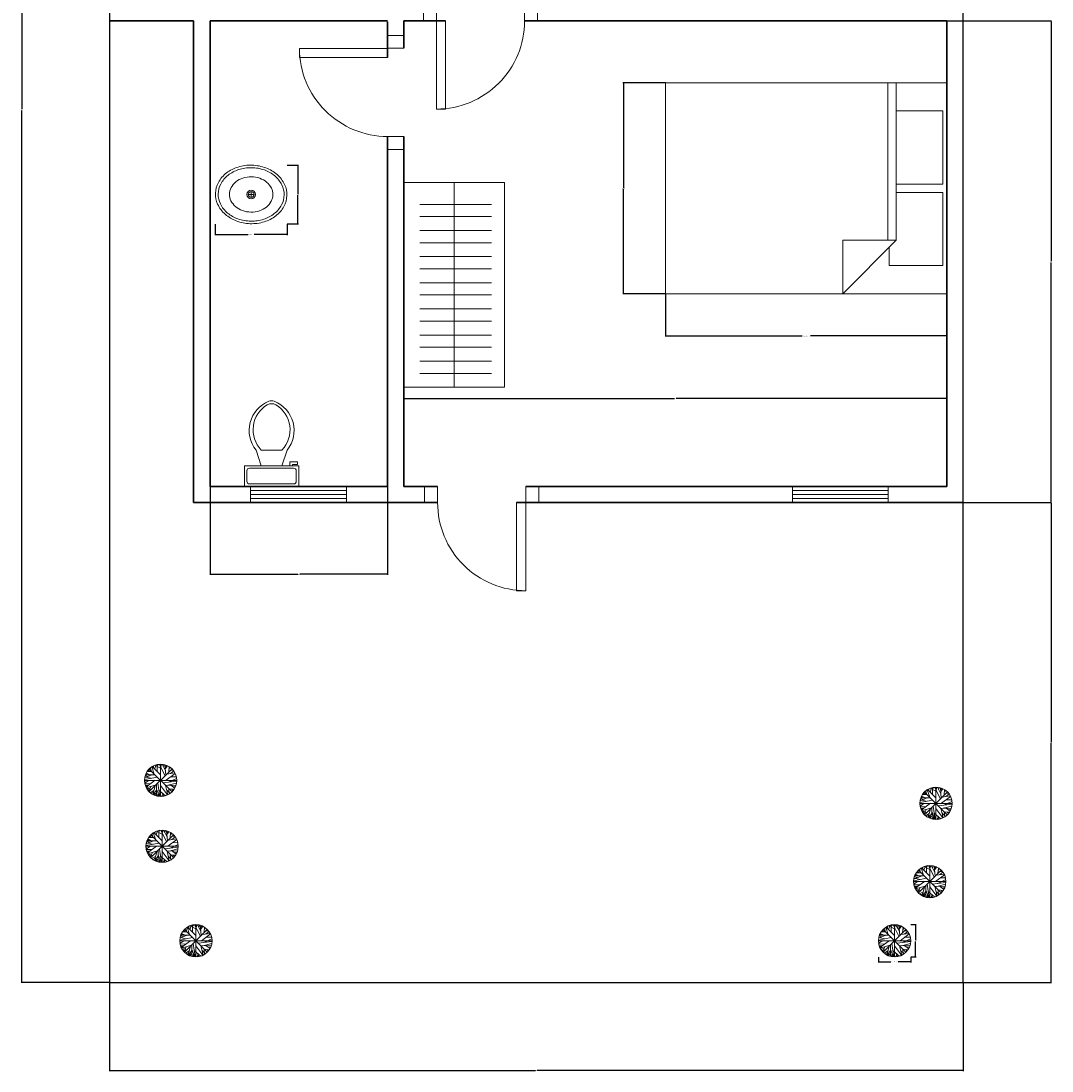
# Model space of a CAD drawing. Units: feet. Extents: x 2306 to 3052, y 829 to 1424.
# Tile 4 of 5: x 2733 to 3052, y 829 to 1154. Entities that reach past the tile are written whole.
import ezdxf

# ---------------------------------------------------------------- set-up
doc = ezdxf.new("R2010")
doc.units = ezdxf.units.FT
for name, color, linetype, lineweight in [('A-ANNO-DIMS', 2, 'Continuous', 18), ('A-DOOR', 3, 'Continuous', 18), ('A-FLOR-FIXT', 9, 'Continuous', 18), ('A-FLOR-OTLN', 7, 'Continuous', 25), ('A-FURN', 8, 'Continuous', 13), ('A-GLAZ', 4, 'Continuous', 18), ('A-WALL', 7, 'Continuous', 35), ('L-PLNT', 94, 'Continuous', 13)]:
    doc.layers.add(name, color=color, linetype=linetype, lineweight=lineweight)
doc.styles.get("Standard").update_dxf_attribs({"font": 'arial.ttf'})
doc.dimstyles.get("Standard").update_dxf_attribs({"dimtxt": 0.18, "dimasz": 0.18, "dimexe": 0.18, "dimexo": 0.0625, "dimgap": 0.09, "dimtad": 0, "dimtih": 1, "dimtoh": 1, "dimdec": 4, "dimzin": 0, "dimdsep": 46, "dimlunit": 4, "dimtxsty": 'Standard', "dimcen": 0.09, "dimadec": 0, "dimazin": 0, "dimtfac": 1, "dimtdec": 4, "dimtofl": 0, "dimtmove": 0, "dimatfit": 3, "dimfxl": 1, "dimtolj": 1, "dimtzin": 0, "dimarcsym": 0})

# ---------------------------------------------------------------- blocks, each defined once
blk = doc.blocks.new('Window - Wood Frame 36 in. Wide plan')
for p, q in [((0, 6), (0, 0)), ((0, 4.5), (36, 4.5)), ((36, 6), (36, 0)), ((0, 3), (36, 3)), ((0, 1.5), (36, 1.5))]:
    blk.add_line(p, q)
blk = doc.blocks.new('Bed - Queen')
for p, q in [((0, -80.00003), (0, 0)), ((0, 0), (59.99999, 0)), ((59.99999, 0), (59.99999, -80.00003)), ((7.99999, -1.2), (28.79998, -1.2)), ((7.99999, -14.4), (7.99999, -1.2)), ((28.79998, -1.2), (28.79998, -14.4)), ((31.19999, -1.2), (51.99999, -1.2)), ((31.19999, -14.4), (31.19999, -1.2)), ((51.99999, -1.2), (51.99999, -16.4)), ((0, -14.4), (44.8, -14.4)), ((59.99999, -29.6), (44.8, -14.4)), ((44.8, -14.4), (44.8, -29.6)), ((44.8, -16.8), (0, -16.8)), ((51.99999, -16.4), (46.79936, -16.4)), ((44.8, -29.6), (59.99999, -29.6)), ((59.99999, -80.00003), (0, -80.00003))]:
    blk.add_line(p, q)
blk = doc.blocks.new('Toilet - top')
for p, q in [((9.5, -6), (9.5, -2)), ((-8, -8.5), (-8, -8)), ((-7, -8), (-7, -9.5)), ((-4, -8), (-6, -14)), ((4, -8), (6, -14)), ((-10, -8.5), (-8, -8.5)), ((-10, -9.5), (-10, -8.5)), ((-7, -9.5), (-10, -9.5)), ((4, -14), (-4, -14))]:
    blk.add_line(p, q)
blk.add_lwpolyline([(10.5, -8), (10.5, 0), (-10.5, 0), (-10.5, -8)], close=True)
for points in [[(-9.5, -2), (-9.5, -6)], [(8.5, -1), (-8.5, -1)], [(-8.5, -7), (8.5, -7)]]:
    blk.add_lwpolyline(points)
for centre, radius, start, end in [((-8.62, -1.88), 0.884, 81.8699, 188.1301), ((8.62, -1.88), 0.884, 351.8699, 98.1301), ((-8.62, -6.12), 0.884, 171.8699, 278.1301), ((8.62, -6.12), 0.884, 261.8699, 8.1301), ((3.52, -21.58), 12.17, 141.4691, 247.9714), ((4.2, -21.82), 11.33, 136.3677, 238.9468), ((-3.52, -21.58), 12.17, 292.0284, 38.5307), ((-4.2, -21.82), 11.33, 301.053, 43.6321), ((0, -27.88), 4, 245.7318, 294.2682), ((0, -29), 4, 254.8605, 285.1395)]:
    blk.add_arc(centre, radius, start, end)
blk = doc.blocks.new('Sink - Oval top')
for p, q in [((-1, 0), (1, 0)), ((0, 1), (0, -1))]:
    blk.add_line(p, q)
for points in [[(-12.23, 0.39, 0.117634), (-11.46, -3.36, 0.104469), (-8.88, -6.8, 0.090016), (-5.08, -9.07, 0.08192), (-0.32, -10.02, 0.08192), (4.49, -9.38, 0.090016), (8.42, -7.36, 0.104469), (11.22, -4.09, 0.117634), (12.23, -0.39, 0.117634), (11.46, 3.36, 0.104469), (8.88, 6.8, 0.090016), (5.08, 9.07, 0.08192), (0.32, 10.02, 0.08192), (-4.49, 9.38, 0.090016), (-8.42, 7.36, 0.104469), (-11.22, 4.09, 0.117634)], [(-11.29, 0.16, 0.118622), (-10.52, -3.25, 0.104678), (-8.07, -6.36, 0.089562), (-4.54, -8.37, 0.081185), (-0.13, -9.15, 0.081185), (4.3, -8.49, 0.089562), (7.89, -6.58, 0.104678), (10.42, -3.55, 0.118622), (11.29, -0.16, 0.118622), (10.52, 3.25, 0.104678), (8.07, 6.36, 0.089562), (4.54, 8.37, 0.081185), (0.13, 9.15, 0.081185), (-4.3, 8.49, 0.089562), (-7.89, 6.58, 0.104678), (-10.42, 3.55, 0.118622)], [(-7.42, 0.08, 0.118283), (-6.91, -2.17, 0.104607), (-5.29, -4.21, 0.089718), (-2.97, -5.53, 0.081436), (-0.07, -6.04, 0.081436), (2.84, -5.59, 0.089718), (5.2, -4.33, 0.104607), (6.86, -2.32, 0.118283), (7.42, -0.08, 0.118283), (6.91, 2.17, 0.104607), (5.29, 4.21, 0.089718), (2.97, 5.53, 0.081436), (0.07, 6.04, 0.081436), (-2.84, 5.59, 0.089718), (-5.2, 4.33, 0.104607), (-6.86, 2.32, 0.118283)]]:
    blk.add_lwpolyline(points, format="xyb", close=True)
for radius in [1.5, 1]:
    blk.add_circle((0, 0), radius)
blk = doc.blocks.new('Tree - deciduous plan')
for p, q in [((-43.8768, 36.4326), (-44.405, 40.2696)), ((42, 42), (-42, -42)), ((42, -42), (-42, 42)), ((-40.1797, 44.558), (-36.4825, 43.2038)), ((-37.0107, 47.0408), (-35.25, 35.5298)), ((-32.6092, 50.4264), (-23.2782, 23.5674)), ((-31.2008, 51.1035), (-0.2149, 20.1818)), ((-26.4472, 46.5894), (-26.2712, 53.8116)), ((-22.0458, 42.0753), (-16.5881, 57.6486)), ((-21.1656, 55.8436), (-0.0388, 45.0094)), ((-12.5388, 54.9406), (-7.9613, 59.4546)), ((-12.3627, 32.1443), (-12.5388, 58.7776)), ((-5.3205, 59.6806), (16.5105, 16.7963)), ((2.426, 54.9406), (-1.4472, 59.9056)), ((0, 59.9996), (0, -60)), ((0.4894, 48.6208), (3.6584, 59.6806)), ((18.2711, 35.5298), (5.419, 59.6806)), ((9.8203, 51.5549), (12.8133, 58.5516)), ((19.6795, 19.5047), (16.3344, 57.6486)), ((17.0387, 51.1035), (23.2006, 55.1666)), ((17.7429, 43.6552), (25.4894, 54.2636)), ((31.6513, 50.8778), (30.2429, 30.5643)), ((31.1232, 42.5267), (35.8767, 48.1693)), ((-59.7219, 2.8025), (-12.0106, 12.0565)), ((-32.2571, 20.6333), (-59.1937, 9.348)), ((-58.6656, 12.7336), (-35.9543, 7.5424)), ((-57.081, 17.9248), (-47.0458, 14.7649)), ((-56.0247, 20.859), (-20.8134, 20.859)), ((-54.7923, 24.4702), (-47.75, 21.0847)), ((-54.6162, -24.7335), (-20.2853, 0.0941)), ((-53.2078, 27.4044), (-40.1797, 20.859)), ((-49.8627, 32.8214), (-32.7853, 32.8214)), ((-45.8134, 38.2383), (-40.5318, 33.0471)), ((54.3626, 25.3731), (20.9119, 0.3198)), ((23.3767, 23.3417), (53.3063, 27.4044)), ((29.3626, -6.6771), (59.4682, 7.091)), ((36.2288, 25.1474), (48.9049, 35.0784)), ((37.1091, 37.1098), (46.6161, 37.5612)), ((38.5175, 13.4107), (58.2359, 13.6364)), ((-60, 0), (60, 0)), ((-59.7219, -4.8714), (-54.2641, -6.6771)), ((-45.2853, -0.1316), (-59.0177, -10.0627)), ((-58.4895, -12.3197), (-36.4825, -11.6426)), ((-57.081, -18.4138), (-45.2853, -17.9624)), ((-52.6797, -18.188), (-55.4966, -22.0251)), ((-53.2078, -27.442), (-16.7641, -16.6081)), ((-38.9472, -29.0219), (-51.4472, -30.6018)), ((-47.2219, -19.3166), (-50.2148, -26.3135)), ((-46.5177, -30.1504), (-49.5106, -33.536)), ((-32.4331, -32.4075), (-48.1021, -35.5674)), ((-43.7008, -34.6645), (-46.6937, -37.373)), ((-35.9543, -22.4765), (-44.0529, -40.5329)), ((-24.6867, -37.8244), (-38.7712, -45.7241)), ((-19.9331, -20.2194), (-28.5599, -52.721)), ((-14.6515, -36.2445), (-27.6797, -52.9467)), ((-14.8275, -15.0282), (-14.6515, -57.6865)), ((-14.6515, -32.1818), (-3.912, -59.4922)), ((-10.074, -10.0627), (-2.5036, -59.7178)), ((-6.2008, -36.2445), (17.919, -57.0094)), ((-0.0388, -19.0909), (25.8415, -53.8495)), ((9.2922, -9.1598), (59.6443, -2.8401)), ((18.6232, -18.6394), (26.7218, -53.3981)), ((18.7992, -18.6394), (57.3556, -17.2853)), ((22.8485, -36.4702), (35.3485, -48.4326)), ((26.3697, -18.4138), (58.9401, -9.8369)), ((30.419, -30.1504), (32.3556, -50.0125)), ((31.4753, -31.279), (49.6091, -33.3103)), ((38.1654, -18.188), (52.426, -29.0219)), ((41.5105, -32.6332), (46.088, -38.0501)), ((45.9119, -24.0564), (55.595, -22.2508)), ((-26.2712, -43.9185), (-34.7219, -48.6583)), ((-14.6515, -47.3041), (-25.0388, -54.3009)), ((-21.5177, -45.4984), (-19.9331, -56.1065)), ((-8.4895, -47.5298), (-11.4825, -58.5893)), ((-6.3768, -52.721), (-9.3698, -58.815)), ((8.4119, -53.1724), (3.8344, -59.4922)), ((5.9471, -46.6269), (10.5246, -58.5893)), ((24.7852, -44.8213), (23.0246, -54.978))]:
    blk.add_line(p, q)
blk.add_circle((0, 0), 60)
blk = doc.blocks.new('DOOR-SWING-STANDARD')
blk.add_lwpolyline([(4.02, 32.25), (4.02, 5), (1.75, 5)])
blk.add_lwpolyline([(4.02, 5), (6.86, 5), (6.86, 32.25), (6.29, 32.25), (4.02, 32.25, -0.414214), (31.27, 5)], format="xyb")
for points in [[(0, 5), (0, 0), (4, 0), (4, 5)], [(31.27, 5), (31.27, 0), (35.27, 0), (35.27, 5)]]:
    blk.add_lwpolyline(points, close=True)
blk = doc.blocks.new('WARDROBE-PLAN')
for p, q in [((0, 0), (0, 63.25)), ((0, 63.25), (8.03, 63.25)), ((2.89, 63.25), (31.17, 63.25)), ((15.59, 0), (15.59, 63.25)), ((31.17, 63.25), (31.17, 0)), ((27.14, 56.53), (4.98, 56.53)), ((27.14, 52.77), (4.98, 52.77)), ((27.14, 48.44), (4.98, 48.44)), ((27.14, 44.68), (4.98, 44.68)), ((27.14, 40.35), (4.98, 40.35)), ((27.14, 36.59), (4.98, 36.59)), ((27.14, 32.26), (4.98, 32.26)), ((27.14, 28.49), (4.98, 28.49)), ((27.14, 24.17), (4.98, 24.17)), ((27.14, 20.4), (4.98, 20.4)), ((27.14, 16.08), (4.98, 16.08)), ((27.14, 12.31), (4.98, 12.31)), ((27.14, 7.99), (4.98, 7.99)), ((27.14, 4.22), (4.98, 4.22)), ((15.59, 4.22), (27.14, 4.22)), ((31.17, 0), (0, 0))]:
    blk.add_line(p, q)
blk = doc.blocks.new('*D18')
at = {"layer": 'A-ANNO-DIMS', "color": 0, "lineweight": -2, "transparency": 16777216}
for p, q in [((2998.3, 864.69), (2998.3, 863.07)), ((3008.3, 864.69), (3008.3, 863.07)), ((2998.48, 863.25), (3002.11, 863.25)), ((3008.12, 863.25), (3004.48, 863.25))]:
    blk.add_line(p, q, dxfattribs=at)
at = {"layer": 'A-ANNO-DIMS', "color": 0, "transparency": 16777216}
for points in [[(2998.48, 863.28), (2998.48, 863.22), (2998.3, 863.25)], [(3008.12, 863.28), (3008.12, 863.22), (3008.3, 863.25)]]:
    blk.add_solid(points, dxfattribs=at)
at = {"layer": 'Defpoints', "color": 0, "transparency": 16777216}
for p in [(2998.3, 864.75), (3008.3, 864.75), (3008.3, 863.25)]:
    blk.add_point(p, dxfattribs=at)
at = {"layer": 'A-ANNO-DIMS', "color": 0, "transparency": 16777216, "insert": (3003.3, 863.25), "char_height": 0.18, "attachment_point": 5}
blk.add_mtext('\\A1;PLANTING 10 TYP.', dxfattribs=at)
blk = doc.blocks.new('*D19')
at = {"layer": 'A-ANNO-DIMS', "color": 0, "lineweight": -2, "transparency": 16777216}
for p, q in [((3008.36, 874.75), (3009.98, 874.75)), ((3009.8, 874.57), (3009.8, 869.93)), ((3009.8, 864.93), (3009.8, 869.57)), ((3008.36, 864.75), (3009.98, 864.75))]:
    blk.add_line(p, q, dxfattribs=at)
at = {"layer": 'A-ANNO-DIMS', "color": 0, "transparency": 16777216}
for points in [[(3009.77, 874.57), (3009.83, 874.57), (3009.8, 874.75)], [(3009.77, 864.93), (3009.83, 864.93), (3009.8, 864.75)]]:
    blk.add_solid(points, dxfattribs=at)
at = {"layer": 'Defpoints', "color": 0, "transparency": 16777216}
for p in [(3008.3, 874.75), (3009.8, 874.75), (3008.3, 864.75)]:
    blk.add_point(p, dxfattribs=at)
at = {"layer": 'A-ANNO-DIMS', "color": 0, "transparency": 16777216, "insert": (3009.8, 869.75), "char_height": 0.18, "attachment_point": 5}
blk.add_mtext('\\A1;10 TYP.', dxfattribs=at)
blk = doc.blocks.new('*D24')
at = {"layer": 'A-ANNO-DIMS', "color": 0, "lineweight": -2, "transparency": 16777216}
for p, q in [((2932.51, 1069.89), (2932.51, 1056.72)), ((3019.52, 1069.89), (3019.52, 1056.72)), ((2932.69, 1056.9), (2974.72, 1056.9)), ((3019.34, 1056.9), (2977.32, 1056.9))]:
    blk.add_line(p, q, dxfattribs=at)
at = {"layer": 'A-ANNO-DIMS', "color": 0, "transparency": 16777216}
for points in [[(2932.69, 1056.93), (2932.69, 1056.87), (2932.51, 1056.9)], [(3019.34, 1056.93), (3019.34, 1056.87), (3019.52, 1056.9)]]:
    blk.add_solid(points, dxfattribs=at)
at = {"layer": 'Defpoints', "color": 0, "transparency": 16777216}
for p in [(2932.51, 1069.95), (3019.52, 1069.95), (3019.52, 1056.9)]:
    blk.add_point(p, dxfattribs=at)
at = {"layer": 'A-ANNO-DIMS', "color": 0, "transparency": 16777216, "insert": (2976.02, 1056.9), "char_height": 0.18, "attachment_point": 5}
blk.add_mtext('\\A1;QUEEN BED 87 TYP.', dxfattribs=at)
blk = doc.blocks.new('*D25')
at = {"layer": 'A-ANNO-DIMS', "color": 0, "lineweight": -2, "transparency": 16777216}
for p, q in [((2932.45, 1135.21), (2919.28, 1135.21)), ((2919.46, 1135.03), (2919.46, 1102.76)), ((2919.46, 1070.13), (2919.46, 1102.4)), ((2932.45, 1069.95), (2919.28, 1069.95))]:
    blk.add_line(p, q, dxfattribs=at)
at = {"layer": 'A-ANNO-DIMS', "color": 0, "transparency": 16777216}
for points in [[(2919.43, 1135.03), (2919.49, 1135.03), (2919.46, 1135.21)], [(2919.43, 1070.13), (2919.49, 1070.13), (2919.46, 1069.95)]]:
    blk.add_solid(points, dxfattribs=at)
at = {"layer": 'Defpoints', "color": 0, "transparency": 16777216}
for p in [(2932.51, 1135.21), (2919.46, 1069.95), (2932.51, 1069.95)]:
    blk.add_point(p, dxfattribs=at)
at = {"layer": 'A-ANNO-DIMS', "color": 0, "transparency": 16777216, "insert": (2919.46, 1102.58), "char_height": 0.18, "attachment_point": 5}
blk.add_mtext('\\A1;65 TYP.', dxfattribs=at)
blk = doc.blocks.new('*D28')
at = {"layer": 'A-ANNO-DIMS', "color": 0, "lineweight": -2, "transparency": 16777216}
for p, q in [((2793.23, 1091.51), (2793.23, 1088.06)), ((2815.41, 1091.51), (2815.41, 1088.06)), ((2793.41, 1088.24), (2803.38, 1088.24)), ((2815.23, 1088.24), (2805.26, 1088.24))]:
    blk.add_line(p, q, dxfattribs=at)
at = {"layer": 'A-ANNO-DIMS', "color": 0, "transparency": 16777216}
for points in [[(2793.41, 1088.27), (2793.41, 1088.21), (2793.23, 1088.24)], [(2815.23, 1088.27), (2815.23, 1088.21), (2815.41, 1088.24)]]:
    blk.add_solid(points, dxfattribs=at)
at = {"layer": 'Defpoints', "color": 0, "transparency": 16777216}
for p in [(2793.23, 1091.57), (2815.41, 1091.57), (2815.41, 1088.24)]:
    blk.add_point(p, dxfattribs=at)
at = {"layer": 'A-ANNO-DIMS', "color": 0, "transparency": 16777216, "insert": (2804.32, 1088.24), "char_height": 0.18, "attachment_point": 5}
blk.add_mtext('\\A1;BASIN 22 TYP.', dxfattribs=at)
blk = doc.blocks.new('*D29')
at = {"layer": 'A-ANNO-DIMS', "color": 0, "lineweight": -2, "transparency": 16777216}
for p, q in [((2815.48, 1109.77), (2818.92, 1109.77)), ((2818.74, 1109.59), (2818.74, 1100.85)), ((2818.74, 1091.75), (2818.74, 1100.49)), ((2815.48, 1091.57), (2818.92, 1091.57))]:
    blk.add_line(p, q, dxfattribs=at)
at = {"layer": 'A-ANNO-DIMS', "color": 0, "transparency": 16777216}
for points in [[(2818.71, 1109.59), (2818.77, 1109.59), (2818.74, 1109.77)], [(2818.71, 1091.75), (2818.77, 1091.75), (2818.74, 1091.57)]]:
    blk.add_solid(points, dxfattribs=at)
at = {"layer": 'Defpoints', "color": 0, "transparency": 16777216}
for p in [(2815.41, 1109.77), (2818.74, 1109.77), (2815.41, 1091.57)]:
    blk.add_point(p, dxfattribs=at)
at = {"layer": 'A-ANNO-DIMS', "color": 0, "transparency": 16777216, "insert": (2818.74, 1100.67), "char_height": 0.18, "attachment_point": 5}
blk.add_mtext('\\A1;18 TYP.', dxfattribs=at)
blk = doc.blocks.new('*D62')
at = {"layer": 'A-ANNO-DIMS', "color": 0, "lineweight": -2, "transparency": 16777216}
for p, q in [((2760.52, 856.76), (2760.52, 829.47)), ((3024.52, 856.76), (3024.52, 829.47)), ((2760.7, 829.65), (2892.23, 829.65)), ((3024.34, 829.65), (2892.81, 829.65))]:
    blk.add_line(p, q, dxfattribs=at)
at = {"layer": 'A-ANNO-DIMS', "color": 0, "transparency": 16777216}
for points in [[(2760.7, 829.68), (2760.7, 829.62), (2760.52, 829.65)], [(3024.34, 829.68), (3024.34, 829.62), (3024.52, 829.65)]]:
    blk.add_solid(points, dxfattribs=at)
at = {"layer": 'Defpoints', "color": 0, "transparency": 16777216}
for p in [(2760.52, 856.83), (3024.52, 856.83), (3024.52, 829.65)]:
    blk.add_point(p, dxfattribs=at)
at = {"layer": 'A-ANNO-DIMS', "color": 0, "transparency": 16777216, "insert": (2892.52, 829.65), "char_height": 0.18, "attachment_point": 5}
blk.add_mtext('\\A1;264', dxfattribs=at)
blk = doc.blocks.new('*D63')
at = {"layer": 'A-ANNO-DIMS', "color": 0, "lineweight": -2, "transparency": 16777216}
for p, q in [((2760.46, 1396.83), (2733.17, 1396.83)), ((2733.35, 1396.65), (2733.35, 1127.01)), ((2733.35, 857.01), (2733.35, 1126.65)), ((2760.46, 856.83), (2733.17, 856.83))]:
    blk.add_line(p, q, dxfattribs=at)
at = {"layer": 'A-ANNO-DIMS', "color": 0, "transparency": 16777216}
for points in [[(2733.32, 1396.65), (2733.38, 1396.65), (2733.35, 1396.83)], [(2733.32, 857.01), (2733.38, 857.01), (2733.35, 856.83)]]:
    blk.add_solid(points, dxfattribs=at)
at = {"layer": 'Defpoints', "color": 0, "transparency": 16777216}
for p in [(2733.35, 1396.83), (2760.52, 1396.83), (2760.52, 856.83)]:
    blk.add_point(p, dxfattribs=at)
at = {"layer": 'A-ANNO-DIMS', "color": 0, "transparency": 16777216, "insert": (2733.35, 1126.83), "char_height": 0.18, "attachment_point": 5}
blk.add_mtext('\\A1;540', dxfattribs=at)
blk = doc.blocks.new('*D64')
at = {"layer": 'A-ANNO-DIMS', "color": 0, "lineweight": -2, "transparency": 16777216}
for p, q in [((3019.59, 1005.33), (3051.88, 1005.33)), ((3051.7, 1005.15), (3051.7, 931.26)), ((3051.7, 857.01), (3051.7, 930.9)), ((3024.59, 856.83), (3051.88, 856.83))]:
    blk.add_line(p, q, dxfattribs=at)
at = {"layer": 'A-ANNO-DIMS', "color": 0, "transparency": 16777216}
for points in [[(3051.67, 1005.15), (3051.73, 1005.15), (3051.7, 1005.33)], [(3051.67, 857.01), (3051.73, 857.01), (3051.7, 856.83)]]:
    blk.add_solid(points, dxfattribs=at)
at = {"layer": 'Defpoints', "color": 0, "transparency": 16777216}
for p in [(3019.52, 1005.33), (3051.7, 1005.33), (3024.52, 856.83)]:
    blk.add_point(p, dxfattribs=at)
at = {"layer": 'A-ANNO-DIMS', "color": 0, "transparency": 16777216, "insert": (3051.7, 931.08), "char_height": 0.18, "attachment_point": 5}
blk.add_mtext('\\A1;148.5', dxfattribs=at)
blk = doc.blocks.new('*D65')
at = {"layer": 'A-ANNO-DIMS', "color": 0, "lineweight": -2, "transparency": 16777216}
for p, q in [((3019.59, 1154.33), (3051.88, 1154.33)), ((3051.7, 1154.15), (3051.7, 1080.01)), ((3051.7, 1005.51), (3051.7, 1079.65)), ((3019.59, 1005.33), (3051.88, 1005.33))]:
    blk.add_line(p, q, dxfattribs=at)
at = {"layer": 'A-ANNO-DIMS', "color": 0, "transparency": 16777216}
for points in [[(3051.67, 1154.15), (3051.73, 1154.15), (3051.7, 1154.33)], [(3051.67, 1005.51), (3051.73, 1005.51), (3051.7, 1005.33)]]:
    blk.add_solid(points, dxfattribs=at)
at = {"layer": 'Defpoints', "color": 0, "transparency": 16777216}
for p in [(3019.52, 1154.33), (3051.7, 1154.33), (3019.52, 1005.33)]:
    blk.add_point(p, dxfattribs=at)
at = {"layer": 'A-ANNO-DIMS', "color": 0, "transparency": 16777216, "insert": (3051.7, 1079.83), "char_height": 0.18, "attachment_point": 5}
blk.add_mtext('\\A1;149', dxfattribs=at)
blk = doc.blocks.new('*D72')
at = {"layer": 'A-ANNO-DIMS', "color": 0, "lineweight": -2, "transparency": 16777216}
for p, q in [((2851.52, 1010.39), (2851.52, 1037.68)), ((2851.7, 1037.5), (2935.24, 1037.5)), ((3019.34, 1037.5), (2935.8, 1037.5)), ((3019.52, 1010.39), (3019.52, 1037.68))]:
    blk.add_line(p, q, dxfattribs=at)
at = {"layer": 'A-ANNO-DIMS', "color": 0, "transparency": 16777216}
for points in [[(2851.7, 1037.53), (2851.7, 1037.47), (2851.52, 1037.5)], [(3019.34, 1037.53), (3019.34, 1037.47), (3019.52, 1037.5)]]:
    blk.add_solid(points, dxfattribs=at)
at = {"layer": 'Defpoints', "color": 0, "transparency": 16777216}
for p in [(3019.52, 1037.5), (2851.52, 1010.33), (3019.52, 1010.33)]:
    blk.add_point(p, dxfattribs=at)
at = {"layer": 'A-ANNO-DIMS', "color": 0, "transparency": 16777216, "insert": (2935.52, 1037.5), "char_height": 0.18, "attachment_point": 5}
blk.add_mtext('\\A1;168', dxfattribs=at)
blk = doc.blocks.new('*D73')
at = {"layer": 'A-ANNO-DIMS', "color": 0, "lineweight": -2, "transparency": 16777216}
for p, q in [((2791.62, 1010.27), (2791.62, 982.97)), ((2846.52, 1010.27), (2846.52, 982.97)), ((2791.8, 983.15), (2818.75, 983.15)), ((2846.34, 983.15), (2819.39, 983.15))]:
    blk.add_line(p, q, dxfattribs=at)
at = {"layer": 'A-ANNO-DIMS', "color": 0, "transparency": 16777216}
for points in [[(2791.8, 983.18), (2791.8, 983.12), (2791.62, 983.15)], [(2846.34, 983.18), (2846.34, 983.12), (2846.52, 983.15)]]:
    blk.add_solid(points, dxfattribs=at)
at = {"layer": 'Defpoints', "color": 0, "transparency": 16777216}
for p in [(2791.62, 1010.33), (2846.52, 1010.33), (2791.62, 983.15)]:
    blk.add_point(p, dxfattribs=at)
at = {"layer": 'A-ANNO-DIMS', "color": 0, "transparency": 16777216, "insert": (2819.07, 983.15), "char_height": 0.18, "attachment_point": 5}
blk.add_mtext('\\A1;54.9', dxfattribs=at)

msp = doc.modelspace()

# ---------------------------------------------------------------- linework, layer by layer
at = {"layer": 'A-DOOR'}
for points in [[(2861.983, 1005.328), (2861.983, 1010.328), (2857.983, 1010.328), (2857.983, 1005.328)], [(2893.254, 1005.328), (2893.254, 1010.328), (2889.254, 1010.328), (2889.254, 1005.328)]]:
    msp.add_lwpolyline(points, close=True, dxfattribs=at)
msp.add_lwpolyline([(2889.237, 1005.328), (2886.398, 1005.328), (2886.398, 978.074), (2886.966, 978.074), (2889.237, 978.074, -0.4142136), (2861.983, 1005.328)], format="xyb", dxfattribs=at)
msp.add_lwpolyline([(2889.237, 978.074), (2889.237, 1005.328), (2891.509, 1005.328)], dxfattribs=at)
at = {"layer": 'A-FLOR-OTLN'}
for p, q in [((2760.523, 1396.827), (2760.523, 856.827)), ((3024.523, 856.827), (3024.523, 1396.827)), ((2760.523, 856.827), (3024.523, 856.827))]:
    msp.add_line(p, q, dxfattribs=at)
at = {"layer": 'A-WALL'}
for p, q in [((2765.523, 1154.328), (2760.523, 1154.328)), ((2786.523, 1154.328), (2765.523, 1154.328)), ((2786.523, 1154.328), (2786.523, 1058.328)), ((2846.523, 1154.328), (2791.618, 1154.328)), ((2791.618, 1154.328), (2791.618, 1010.328)), ((2846.523, 1143.019), (2846.523, 1154.102)), ((2851.523, 1154.328), (2851.523, 1145.875)), ((2864.452, 1154.328), (2851.523, 1154.328)), ((2864.452, 1154.328), (2851.523, 1154.328)), ((2907.023, 1154.328), (2888.867, 1154.328)), ((3019.523, 1154.328), (2888.867, 1154.328)), ((2907.023, 1154.328), (3019.523, 1154.328)), ((3019.523, 1099.327), (3019.523, 1154.328)), ((2846.523, 1039.102), (2846.523, 1118.604)), ((2851.523, 1118.604), (2851.523, 1010.328)), ((3019.523, 1099.327), (3019.523, 1094.327)), ((3019.523, 1010.328), (3019.523, 1094.327)), ((2786.523, 1058.328), (2786.523, 1005.328)), ((2846.523, 1039.102), (2846.523, 1010.328)), ((2846.523, 1010.328), (2791.618, 1010.328)), ((2851.523, 1010.328), (2861.983, 1010.328)), ((2889.254, 1010.328), (3019.523, 1010.328)), ((2928.523, 1010.328), (3019.523, 1010.328)), ((2846.523, 1005.328), (2786.523, 1005.328)), ((2861.983, 1005.328), (2846.523, 1005.328)), ((2928.523, 1005.328), (2886.398, 1005.328)), ((2928.523, 1005.328), (3019.523, 1005.328)), ((3019.523, 1005.328), (3024.523, 1005.328))]:
    msp.add_line(p, q, dxfattribs=at)

# ---------------------------------------------------------------- block references
at = {"layer": 'A-DOOR', "extrusion": (0, 0, -1), "zscale": -1}
for p, rotation in [((-2857.597, 1159.328), 180), ((-2851.523, 1149.875), 269.9999999999983)]:
    msp.add_blockref('DOOR-SWING-STANDARD', p, dxfattribs=dict(at, rotation=rotation))
at = {"layer": 'A-FLOR-FIXT', "xscale": 0.9036611704051442, "yscale": 0.9036611704051442, "zscale": 0.9036611704051442}
msp.add_blockref('Sink - Oval top', (2804.321, 1100.67), dxfattribs=at)
at = {"layer": 'A-FLOR-FIXT', "xscale": 0.8023769030949434, "yscale": 0.8023769030949434, "zscale": 0.8023769030949434, "rotation": 180}
msp.add_blockref('Toilet - top', (2810.645, 1010.328), dxfattribs=at)
at = {"layer": 'A-FURN', "xscale": 1.087596012527482, "yscale": 1.087596012527482, "zscale": 1.087596012527482, "rotation": 270}
msp.add_blockref('Bed - Queen', (3019.523, 1135.208), dxfattribs=at)
at = {"layer": 'A-FURN'}
msp.add_blockref('WARDROBE-PLAN', (2851.522, 1041.067), dxfattribs=at)
at = {"layer": 'A-GLAZ', "xscale": 0.82338841385576, "yscale": 0.82338841385576, "zscale": 0.82338841385576}
for p in [(2804.141, 1005.387), (2971.726, 1005.387)]:
    msp.add_blockref('Window - Wood Frame 36 in. Wide plan', p, dxfattribs=at)
at = {"layer": 'L-PLNT', "xscale": 0.0833333333333333, "yscale": 0.0833333333333333, "zscale": 0.0833333333333333}
for p in [(2776.308, 919.395), (3016.118, 912.277), (2776.783, 898.992), (3014.219, 888.078), (2787.23, 869.751), (3003.297, 869.751)]:
    msp.add_blockref('Tree - deciduous plan', p, dxfattribs=at)

# ---------------------------------------------------------------- dimensions: what is measured, and where the dimension line sits
at = {"layer": 'A-ANNO-DIMS'}
for base, p1, p2, angle, override, picture, middle in [((2733.348, 1396.827), (2760.523, 856.827), (2760.523, 1396.827), 90, {"dimdec": 0, "dimlfac": 1, "dimrnd": 0, "dimzin": 0, "dimdsep": 46, "dimlunit": 2}, '*D63', (2733.348, 1126.827)), ((3051.698, 1154.328), (3019.523, 1005.328), (3019.523, 1154.328), 90, {"dimdec": 0, "dimlfac": 1, "dimrnd": 0, "dimzin": 0, "dimdsep": 46, "dimlunit": 2}, '*D65', (3051.698, 1079.828)), ((2791.618, 983.153), (2846.523, 1010.328), (2791.618, 1010.328), 180, {"dimdec": 1, "dimlfac": 1, "dimrnd": 0, "dimzin": 0, "dimdsep": 46, "dimlunit": 2}, '*D73', (2819.07, 983.153)), ((3051.698, 1005.328), (3024.523, 856.827), (3019.523, 1005.328), 90, {"dimdec": 1, "dimlfac": 1, "dimrnd": 0, "dimzin": 0, "dimdsep": 46, "dimlunit": 2}, '*D64', (3051.698, 931.078))]:
    dim = msp.add_linear_dim(base=base, p1=p1, p2=p2, angle=angle, dimstyle='Standard', override=override, dxfattribs=at)
    dim.commit()
    dim.dimension.update_dxf_attribs({"geometry": picture, "text_midpoint": middle})
for base, p1, p2, angle, picture, middle in [((2919.464, 1069.952), (2932.515, 1135.208), (2932.515, 1069.952), 270, '*D25', (2919.464, 1102.58)), ((2818.741, 1109.768), (2815.414, 1091.571), (2815.414, 1109.768), 90, '*D29', (2818.741, 1100.67)), ((3009.797, 874.751), (3008.297, 864.751), (3008.297, 874.751), 90, '*D19', (3009.797, 869.751))]:
    dim = msp.add_linear_dim(base=base, p1=p1, p2=p2, angle=angle, text='<> TYP.', dimstyle='Standard', override={"dimdec": 0, "dimlfac": 1, "dimrnd": 0, "dimzin": 0, "dimdsep": 46, "dimlunit": 2}, dxfattribs=at)
    dim.commit()
    dim.dimension.update_dxf_attribs({"geometry": picture, "text_midpoint": middle})
for base, p1, p2, text, picture, middle in [((2815.414, 1088.244), (2793.228, 1091.571), (2815.414, 1091.571), 'BASIN <> TYP.', '*D28', (2804.321, 1088.244)), ((3019.523, 1056.901), (2932.515, 1069.952), (3019.523, 1069.952), 'QUEEN BED <> TYP.', '*D24', (2976.019, 1056.901)), ((3008.297, 863.251), (2998.297, 864.751), (3008.297, 864.751), 'PLANTING <> TYP.', '*D18', (3003.297, 863.251))]:
    dim = msp.add_linear_dim(base=base, p1=p1, p2=p2, text=text, dimstyle='Standard', override={"dimdec": 0, "dimlfac": 1, "dimrnd": 0, "dimzin": 0, "dimdsep": 46, "dimlunit": 2}, dxfattribs=at)
    dim.commit()
    dim.dimension.update_dxf_attribs({"geometry": picture, "text_midpoint": middle})
for base, p1, p2, picture, middle in [((3019.523, 1037.503), (2851.523, 1010.328), (3019.523, 1010.328), '*D72', (2935.523, 1037.503)), ((3024.523, 829.652), (2760.523, 856.827), (3024.523, 856.827), '*D62', (2892.523, 829.652))]:
    dim = msp.add_linear_dim(base=base, p1=p1, p2=p2, dimstyle='Standard', override={"dimdec": 0, "dimlfac": 1, "dimrnd": 0, "dimzin": 0, "dimdsep": 46, "dimlunit": 2}, dxfattribs=at)
    dim.commit()
    dim.dimension.update_dxf_attribs({"geometry": picture, "text_midpoint": middle})

doc.saveas('drawing.dxf')
